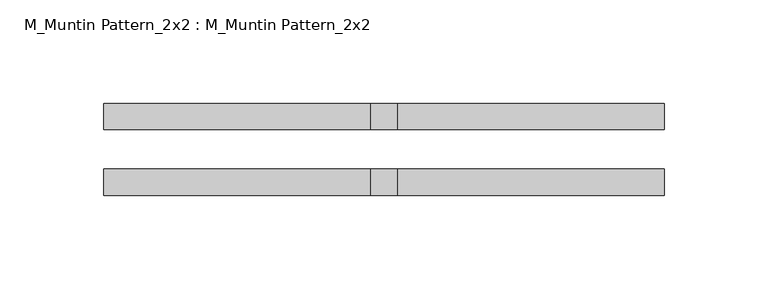
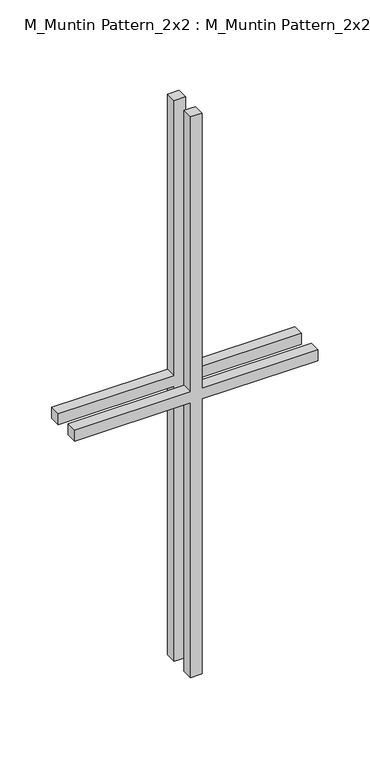
"""IFC4 building model written with IfcOpenShell, lengths in millimetres: proxy geometry, M_Muntin Pattern_2x2 : M_Muntin Pattern_2x2."""

from ifc_helpers import new_model, si_unit, frame, origin, place, context, project, spatial, polyline, outline, extrude, source, transform, mapped, element, save


def m_muntin_pattern_2x2_m_muntin_pattern_2x2_777d393c(model_context):
    return source(origin(), model_context, "Body", "SweptSolid", [
        extrude(outline(polyline([(336.5, -6.35), (336.5, -135.4666667), (323.8, -135.4666667), (323.8, -6.35), (0.0, -6.35), (0.0, 6.35), (323.8, 6.35), (323.8, 135.4666667), (336.5, 135.4666667), (336.5, 6.35), (660.3, 6.35), (660.3, -6.35), (336.5, -6.35)])), frame((0.0, 9.525, 0.0), z_axis=(0.0, 1.0, 0.0), x_axis=(0.0, 0.0, 1.0)), (0.0, 0.0, 1.0), 12.7),
        extrude(outline(polyline([(336.5, -6.35), (336.5, -135.4666667), (323.8, -135.4666667), (323.8, -6.35), (0.0, -6.35), (0.0, 6.35), (323.8, 6.35), (323.8, 135.4666667), (336.5, 135.4666667), (336.5, 6.35), (660.3, 6.35), (660.3, -6.35), (336.5, -6.35)])), frame((0.0, -22.225, 0.0), z_axis=(0.0, 1.0, 0.0), x_axis=(0.0, 0.0, 1.0)), (0.0, 0.0, 1.0), 12.7),
    ])


if __name__ == "__main__":
    model = new_model("IFC4")
    model_context = context("Model", 3, world=origin())
    ifc_project = project(units=[si_unit("LENGTHUNIT", "METRE", prefix="MILLI")], contexts=[model_context])
    site = spatial("IfcSite", under=ifc_project)
    building = spatial("IfcBuilding", under=site)
    placement = place(None, origin())
    m_muntin_pattern_2x2_m_muntin_pattern_2x2_shape = m_muntin_pattern_2x2_m_muntin_pattern_2x2_777d393c(model_context)
    element("IfcBuildingElementProxy", 1, Name="M_Muntin Pattern_2x2 : M_Muntin Pattern_2x2", ObjectType="M_Muntin Pattern_2x2 : M_Muntin Pattern_2x2", at=placement, inside=building, context=model_context, shape_type="MappedRepresentation", body=[
        mapped(m_muntin_pattern_2x2_m_muntin_pattern_2x2_shape, transform((0.0, 0.0, 0.0), x_axis=(1.0, 0.0, 0.0), y_axis=(0.0, 1.0, 0.0), z_axis=(0.0, 0.0, 1.0))),
    ])
    save(model, "model.ifc")

# Revit data of these elements
# Type "M_Muntin Pattern_2x2 : M_Muntin Pattern_2x2"
#   Width [instance default] = 3' - 11.24409"
#   Thickness = 0' - 0 1/2"
#   Height [instance default] = 3' - 11.24409"
#   Distance = 0' - 0 3/4"
#   Interior Material [instance default] = none
#   Exterior Material [instance default] = none
#   Default Elevation = 0
# Element 1 (IfcBuildingElementProxy, "M_Muntin Pattern_2x2 : M_Muntin Pattern_2x2")
#   Width = 0' - 10.66667"
#   Height = 2' - 1.99606"
#   Interior Material = Wood - Stained
#   Exterior Material = Clad - White
#   Materials on its faces: "Clad - White", "Wood - Stained"
# Materials
#   "Clad - White": class "Wood", colour RGB 242 242 238, transparency 0, Cost = 0
#   "Wood - Stained": class "Wood", colour RGB 224 178 126, transparency 0, Cost = 0
